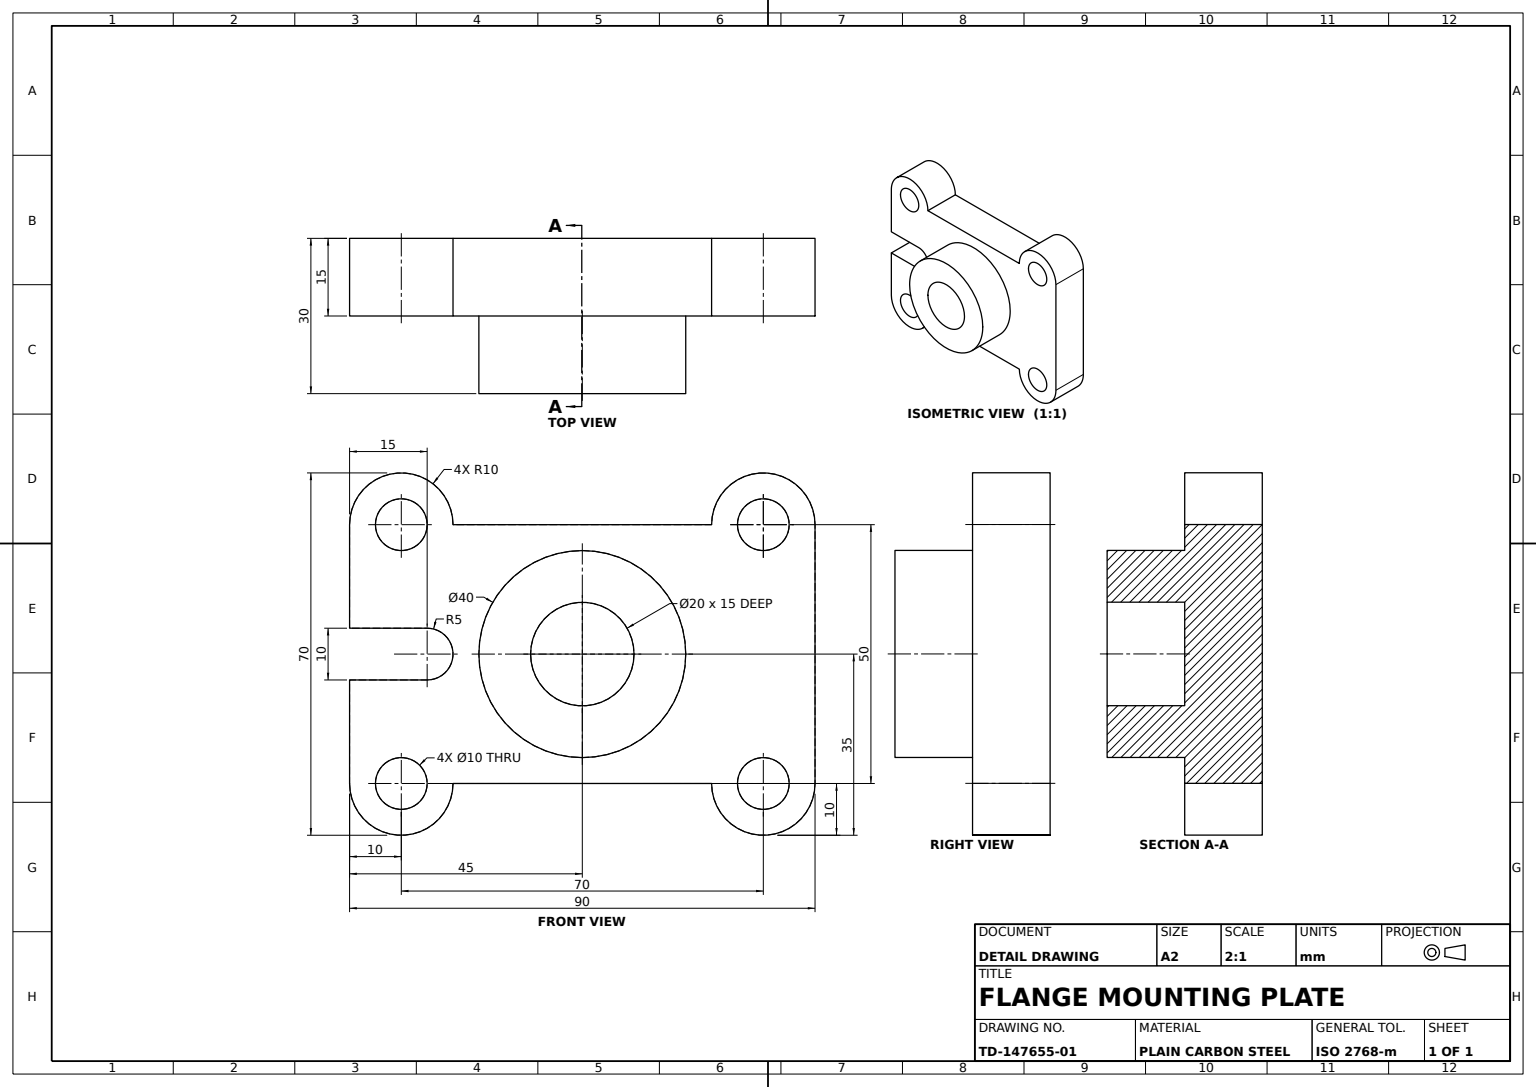
from build123d import *

# Parameters (mm, degrees)
FLANGE_PLATE_DEPTH     = 15
SIDE_NOTCH_SKETCH_R    = 5
SIDE_NOTCH_10X10_DEPTH = 15
HUB_BOSS_SKETCH_R      = 20
HUB_BOSS_40_DEPTH      = 15
BORE_SKETCH_R          = 10
BORE_20_DEPTH          = 15


with BuildPart() as part:
    # Flange Plate Profile Sketch → Flange Plate (new body)
    with BuildSketch(Plane.XY):
        with BuildLine():
            Line((9.999999107, -5.133e-06), (59.999999107, -5.133e-06))
            ThreePointArc((59.999999107, -5.133e-06), (69.999996541, 10), (79.999999107, 0))
            Line((79.999999107, 0), (79.999999107, -50))
            ThreePointArc((79.999999107, -50), (70.000001674, -60), (59.999999107, -50.000005133))
            Line((59.999999107, -50.000005133), (10.000000893, -50.000005133))
            ThreePointArc((10.000000893, -50.000005133), (1.674e-06, -60.000006696), (-9.999999107, -50.000006696))
            Line((-9.999999107, -50.000006696), (-9.999999107, -30))
            Line((-9.999999107, -30), (5.000000893, -30))
            ThreePointArc((5.000000893, -30), (10.000001691, -25.000000893), (5.000002678, -20))
            Line((5.000002678, -20), (-9.999999107, -20))
            Line((-9.999999107, -20), (-9.999999107, 0))
            ThreePointArc((-9.999999107, 0), (2.567e-06, 9.999999107), (9.999999107, -5.133e-06))
        make_face()
    extrude(amount=FLANGE_PLATE_DEPTH)

    # Side Notch Sketch → Side Notch 10x10 (cut)
    with BuildSketch(Plane.XY.offset(15)):
        Circle(SIDE_NOTCH_SKETCH_R)
        with Locations((69.999999107, 0)):
            Circle(SIDE_NOTCH_SKETCH_R)
        with Locations((69.999999107, -50)):
            Circle(SIDE_NOTCH_SKETCH_R)
        with Locations((8.93e-07, -50.000006696)):
            Circle(SIDE_NOTCH_SKETCH_R)
    extrude(amount=-SIDE_NOTCH_10X10_DEPTH, mode=Mode.SUBTRACT)

    # Hub Boss Sketch → Hub Boss Ø40 (add)
    with BuildSketch(Plane.XY.offset(15)):
        with Locations((34.999999107, -25.000005133)):
            Circle(HUB_BOSS_SKETCH_R)
    extrude(amount=HUB_BOSS_40_DEPTH)

    # Bore Sketch → Bore Ø20 (cut)
    with BuildSketch(Plane.XY.offset(30)):
        with Locations((34.999999107, -25.000005133)):
            Circle(BORE_SKETCH_R)
    extrude(amount=-BORE_20_DEPTH, mode=Mode.SUBTRACT)


solid = part.part
